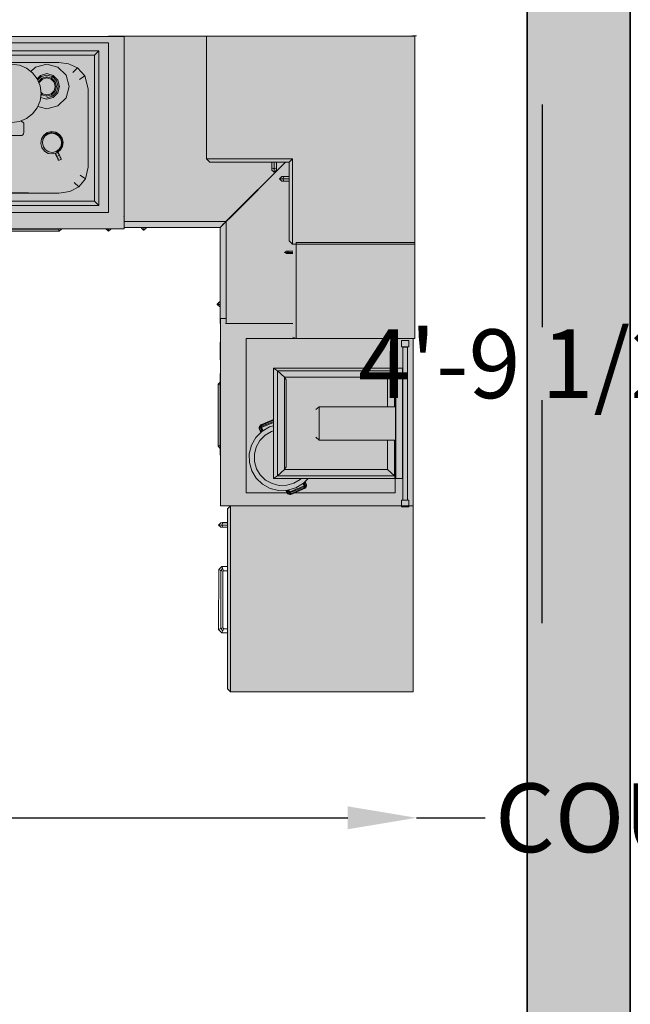
# Model space of a CAD drawing. Units: inches. Extents: x 2178 to 3409, y 1711 to 2279.
# Tile 6 of 8: x 2423 to 2476, y 2140 to 2226. Entities that reach past the tile are written whole.
import ezdxf

# ---------------------------------------------------------------- set-up
doc = ezdxf.new("R2010")
doc.units = ezdxf.units.IN
for name, color, linetype, lineweight in [('A-ANNO-DIMS', 2, 'Continuous', 18), ('A-FLOR-FIXT', 8, 'Continuous', 18), ('A-WALL', 7, 'Continuous', 35), ('A-WALL-PATT', 252, 'Continuous', 13)]:
    doc.layers.add(name, color=color, linetype=linetype, lineweight=lineweight)
doc.layers.add('hatch', color=254, linetype='Continuous')
doc.styles.get("Standard").update_dxf_attribs({"font": 'arial.ttf'})
doc.dimstyles.get("Standard").update_dxf_attribs({"dimtxt": 6, "dimasz": 6, "dimexe": 0.18, "dimexo": 0.0625, "dimgap": 0.09, "dimtad": 0, "dimtih": 1, "dimtoh": 1, "dimdec": 4, "dimzin": 0, "dimdsep": 46, "dimlunit": 4, "dimtxsty": 'Standard', "dimcen": 0.09, "dimse1": 1, "dimse2": 1, "dimadec": 0, "dimazin": 0, "dimtfac": 1, "dimtdec": 4, "dimtofl": 0, "dimtmove": 0, "dimatfit": 3, "dimfxl": 1, "dimtolj": 1, "dimtzin": 0, "dimarcsym": 0})

# ---------------------------------------------------------------- blocks, each defined once
blk = doc.blocks.new('kithen1')
at = {"layer": 'hatch'}
blk.add_hatch(color=256, dxfattribs=at).paths.add_polyline_path([(-2799.7, -8.3), (-2273.3, -8.3), (-2273.3, -1.7), (-2257.5, -1.7), (-2257.5, -1.1), (-1023.7, -1.1), (-1023.7, 0), (0, 0), (0, -0.3), (0.3, -0.3), (0.3, -1009.9), (-6.1, -1009.9), (-6.1, -2189.3), (-615.8, -2189.3), (-626.5, -2178.9), (-626.5, -1578.2), (-615.8, -1567.8), (-649.5, -1567.8), (-649.5, -1399.1), (-650.3, -1399.1), (-650.3, -1376.8), (-657.9, -1368.5), (-657.8, -1162.4), (-650.3, -1155.1), (-650.3, -1126.4), (-649.5, -1126.4), (-649.5, -1081.1), (-650.3, -1081.1), (-650.3, -1021.1), (-649.5, -1021.1), (-649.5, -959.1), (-651, -959.1), (-650.7, -903), (-653.5, -903), (-660.6, -895.5), (-660.5, -894.6), (-653.5, -887.1), (-651, -887.1), (-651, -638.7), (-651.2, -638.5), (-898.3, -638.5), (-898.3, -640.4), (-905.9, -647.4), (-906.8, -647.4), (-914.3, -640.4), (-914.3, -638.5), (-971.4, -638.5), (-971.4, -642.6), (-1016.2, -642.6), (-1016.2, -643.9), (-1023.8, -650.9), (-1024.7, -650.9), (-1032.2, -643.9), (-1032.2, -642.6), (-1179.7, -642.6), (-1188.8, -650.9), (-1395.6, -650.9), (-1403.7, -642.6), (-1813.5, -642.6), (-1822.6, -650.9), (-2029.4, -650.9), (-2037.5, -642.6), (-2257.5, -642.6), (-2257.5, -618.1), (-2261.3, -618.1), (-2271.7, -628.7), (-2458, -628.7), (-2727.7, -628.7), (-2727.7, -651.1), (-2735, -658.1), (-2735.9, -658), (-2743.2, -651.1), (-2743.2, -628.7), (-2789.4, -628.7), (-2799.7, -618.1)])
at = {"color": 0}
for p, q in [((0, 0), (-1023.7, 0)), ((-696.5, 0), (-696.5, -409.2)), ((-8.6, 1.9), (-10.5, 0)), ((-10.1, 0), (-8.2, 1.9)), ((-8.2, 1.9), (-8.3, 1.8)), ((-8.3, 1.9), (-8.3, 0)), ((5.4, 1.8), (-8.3, 1.8)), ((0, 0), (0, -694.7)), ((0, -0.3), (0, 0)), ((-2261.3, -8.3), (-2799.7, -8.3)), ((-2799.7, -8.3), (-2799.7, -618.1)), ((-2273.3, -1.9), (-2273.9, -1.9)), ((-2273.9, -1.9), (-2273.9, -8.3)), ((-2261.3, -1.7), (-2273.3, -1.7)), ((-2273.3, -1.7), (-2273.3, -8.3)), ((-2261.3, -601.6), (-2261.3, -1.7)), ((-2261.3, -618.1), (-2261.3, -8.3)), ((-2261, -8.5), (-2261.3, -8.5)), ((-971.4, -1.1), (-2257.5, -1.1)), ((-2257.5, -1.1), (-2257.5, -642.6)), ((-1023.7, -22.5), (-2210.1, -22.5)), ((-2210.1, -22.5), (-2210.1, -589.1)), ((-1023.7, -589.1), (-1023.7, -22.5)), ((-971.4, -1.1), (-971.4, -600.9)), ((0.3, -0.3), (0, -0.3)), ((0.3, -671.1), (0.3, -0.3)), ((-2257.5, -51.5), (-2261.3, -51.5)), ((-2261.3, -51.5), (-2261.3, -536.3)), ((-2183.7, -48.8), (-1056.9, -48.9)), ((-2169.4, -62.7), (-2183.7, -48.8)), ((-2183.7, -48.8), (-2183.7, -565)), ((-2169.7, -550.2), (-2169.4, -62.7)), ((-1071, -63.6), (-2169.4, -62.7)), ((-1056.9, -48.9), (-1071, -63.6)), ((-1071, -550.2), (-1071, -63.6)), ((-1056.9, -48.9), (-1056.9, -565)), ((-2136.6, -97.6), (-2156.1, -126.2)), ((-2103.6, -76.6), (-2136.6, -97.6)), ((-2135.1, -98.9), (-2102.3, -78.1)), ((-2100.1, -80.6), (-2132.5, -101.2)), ((-2093.2, -88.3), (-2124.5, -108.2)), ((-2057.7, -68.5), (-2103.6, -76.6)), ((-2102.3, -78.1), (-2056.8, -70)), ((-2100.1, -80.6), (-2102.3, -78.1)), ((-2055, -72.6), (-2100.1, -80.6)), ((-2093.2, -88.3), (-2100.1, -80.6)), ((-2049.7, -80.6), (-2093.2, -88.3)), ((-1740.9, -68.5), (-2057.7, -68.5)), ((-2056.8, -70), (-1741.9, -70)), ((-1743.7, -72.6), (-2055, -72.6)), ((-1749, -80.6), (-2049.7, -80.6)), ((-1716.2, -84.8), (-1749, -80.6)), ((-1709.7, -76.9), (-1743.7, -72.6)), ((-1741.9, -70), (-1707.6, -74.4)), ((-1706.4, -72.9), (-1740.9, -68.5)), ((-1685.6, -98.8), (-1716.2, -84.8)), ((-1678, -91.5), (-1709.7, -76.9)), ((-1707.6, -74.4), (-1675.5, -89.1)), ((-1674.1, -87.7), (-1706.4, -72.9)), ((-1678, -91.5), (-1685.6, -98.8)), ((-1651.9, -119.5), (-1678, -91.5)), ((-1675.5, -89.1), (-1649.1, -117.4)), ((-1647.6, -116.2), (-1674.1, -87.7)), ((-1523.7, -95.6), (-1554, -114.9)), ((-1481.5, -88.1), (-1523.7, -95.6)), ((-1523.7, -95.6), (-1509.8, -111.1)), ((-1189.8, -88.1), (-1481.5, -88.1)), ((-1396, -106.6), (-1372.5, -96.9)), ((-1372.5, -96.9), (-1347.3, -93.6)), ((-1347.3, -93.6), (-1322, -96.9)), ((-1322, -96.9), (-1298.5, -106.6)), ((-1268.1, -102.9), (-1230.5, -92.9)), ((-1230.5, -92.9), (-1193, -102.9)), ((-1157.9, -92.2), (-1189.8, -88.1)), ((-1128.2, -105.8), (-1157.9, -92.2)), ((-2156.1, -126.2), (-2163.3, -163.2)), ((-2161.7, -164.1), (-2154.5, -127.3)), ((-2151.7, -129.3), (-2158.8, -165.7)), ((-2154.5, -127.3), (-2135.1, -98.9)), ((-2151.7, -129.3), (-2154.5, -127.3)), ((-2132.5, -101.2), (-2151.7, -129.3)), ((-2143, -135.3), (-2151.7, -129.3)), ((-2124.5, -108.2), (-2143, -135.3)), ((-2132.5, -101.2), (-2135.1, -98.9)), ((-2124.5, -108.2), (-2132.5, -101.2)), ((-1685.6, -98.8), (-1660.4, -125.8)), ((-1660.4, -125.8), (-1651.9, -119.5)), ((-1648.8, -170.4), (-1660.4, -125.8)), ((-1649.1, -117.4), (-1651.9, -119.5)), ((-1651.9, -119.5), (-1639.9, -165.7)), ((-1649.1, -117.4), (-1637, -164.1)), ((-1635.3, -163.2), (-1647.6, -116.2)), ((-1554, -114.9), (-1572, -141.2)), ((-1431.7, -142.2), (-1416.2, -122.1)), ((-1416.2, -122.1), (-1396, -106.6)), ((-1298.5, -106.6), (-1278.3, -122.1)), ((-1283.4, -118.2), (-1268.1, -102.9)), ((-1278.3, -122.1), (-1262.8, -142.2)), ((-1252, -130.7), (-1263.1, -141.8)), ((-1252, -130.7), (-1230.5, -124.9)), ((-1249.5, -134.9), (-1230.5, -129.8)), ((-1230.5, -124.9), (-1209.1, -130.7)), ((-1230.5, -129.8), (-1211.6, -134.9)), ((-1209.1, -130.7), (-1193.4, -146.3)), ((-1193, -102.9), (-1165.5, -130.3)), ((-1165.5, -130.3), (-1155.5, -167.7)), ((-1143.5, -120.5), (-1128.2, -105.8)), ((-1128.2, -105.8), (-1103.8, -132)), ((-2163.3, -163.2), (-2163.3, -447.5)), ((-2161.7, -446.6), (-2161.7, -164.1)), ((-2149.9, -170.5), (-2143, -135.3)), ((-1637, -164.1), (-1637, -446.6)), ((-1635.3, -447.4), (-1635.3, -163.2)), ((-1572, -141.2), (-1578.6, -175.3)), ((-1572, -141.2), (-1554.6, -153.3)), ((-1441.5, -165.7), (-1431.7, -142.2)), ((-1262.8, -142.2), (-1253, -165.7)), ((-1249.5, -134.9), (-1261, -146.4)), ((-1258.4, -151.7), (-1258.6, -152.3)), ((-1246.6, -139.9), (-1258.4, -151.7)), ((-1255.2, -153.5), (-1258.4, -151.7)), ((-1255.2, -153.5), (-1256.4, -157.6)), ((-1244.8, -143), (-1255.2, -153.5)), ((-1230.5, -135.6), (-1246.6, -139.9)), ((-1246.6, -139.9), (-1244.8, -143)), ((-1244.8, -143), (-1230.5, -139.2)), ((-1214.5, -139.9), (-1230.5, -135.6)), ((-1230.5, -135.6), (-1230.5, -139.2)), ((-1230.5, -139.2), (-1216.3, -143)), ((-1216.3, -143), (-1214.5, -139.9)), ((-1205.8, -153.5), (-1216.3, -143)), ((-1211.6, -134.9), (-1214.5, -139.9)), ((-1214.5, -139.9), (-1202.7, -151.7)), ((-1211.6, -134.9), (-1197.7, -148.8)), ((-1202.7, -151.7), (-1205.8, -153.5)), ((-1205.8, -153.5), (-1202, -167.7)), ((-1198.4, -167.7), (-1202.7, -151.7)), ((-1197.7, -148.8), (-1192.6, -167.7)), ((-1193.4, -146.3), (-1187.6, -167.7)), ((-1103.8, -132), (-1120.8, -144.8)), ((-1103.8, -132), (-1092.5, -175.3)), ((-2158.8, -165.7), (-2158.8, -445)), ((-2149.9, -440.2), (-2149.9, -170.5)), ((-1648.8, -440.2), (-1648.8, -170.4)), ((-1639.9, -165.7), (-1639.9, -445)), ((-1578.6, -175.3), (-1578.6, -437)), ((-1444.8, -190.8), (-1441.5, -165.7)), ((-1441.5, -216), (-1444.8, -190.8)), ((-1253, -165.7), (-1249.7, -190.8)), ((-1249.7, -190.8), (-1253, -216)), ((-1250.2, -186.9), (-1244.8, -192.3)), ((-1246.6, -195.5), (-1249.9, -192.2)), ((-1244.8, -192.3), (-1246.6, -195.5)), ((-1230.5, -199.7), (-1246.6, -195.5)), ((-1230.5, -196.1), (-1244.8, -192.3)), ((-1216.3, -192.3), (-1230.5, -196.1)), ((-1214.5, -195.5), (-1230.5, -199.7)), ((-1230.5, -196.1), (-1230.5, -199.7)), ((-1205.8, -181.9), (-1216.3, -192.3)), ((-1216.3, -192.3), (-1214.5, -195.5)), ((-1214.5, -195.5), (-1202.7, -183.7)), ((-1211.6, -200.5), (-1214.5, -195.5)), ((-1197.7, -186.6), (-1211.6, -200.5)), ((-1193.4, -189.1), (-1209.1, -204.7)), ((-1202, -167.7), (-1205.8, -181.9)), ((-1205.8, -181.9), (-1202.7, -183.7)), ((-1202.7, -183.7), (-1198.4, -167.7)), ((-1202, -167.7), (-1198.4, -167.7)), ((-1192.6, -167.7), (-1197.7, -186.6)), ((-1187.6, -167.7), (-1193.4, -189.1)), ((-1155.5, -167.7), (-1165.5, -205.1)), ((-1092.5, -175.3), (-1092.5, -437)), ((-1442, -212), (-1442.1, -213.6)), ((-1442.1, -213.6), (-1441.9, -216.3)), ((-1441.9, -216.3), (-1441.5, -218.2)), ((-1431.7, -239.4), (-1441.5, -216)), ((-1441.5, -218.2), (-1440.8, -218.9)), ((-1440.8, -218.9), (-1440.3, -218.9)), ((-1253, -216), (-1262.8, -239.4)), ((-1230.5, -210.4), (-1251.6, -204.8)), ((-1250.8, -199.1), (-1249.5, -200.5)), ((-1211.6, -200.5), (-1230.5, -205.5)), ((-1209.1, -204.7), (-1230.5, -210.4)), ((-1165.5, -205.1), (-1193, -232.5)), ((-1416.2, -259.6), (-1431.7, -239.4)), ((-1396, -275), (-1416.2, -259.6)), ((-1278.3, -259.6), (-1298.5, -275)), ((-1262.8, -239.4), (-1278.3, -259.6)), ((-1230.5, -242.5), (-1260.7, -234.4)), ((-1193, -232.5), (-1230.5, -242.5)), ((-1914.6, -272.1), (-1926.9, -292)), ((-1926.9, -292), (-1921.4, -314.8)), ((-1891.8, -266.6), (-1914.6, -272.1)), ((-1871.8, -278.8), (-1891.8, -266.6)), ((-1866.3, -301.6), (-1871.8, -278.8)), ((-1493.1, -302.1), (-1453.2, -294.2)), ((-1453.2, -294.3), (-1493.1, -302.2)), ((-1453.2, -294.2), (-1413.4, -302.1)), ((-1413.4, -302.2), (-1453.2, -294.3)), ((-1453.2, -294.3), (-1453.2, -296.5)), ((-1372.5, -284.8), (-1396, -275)), ((-1347.3, -288.1), (-1372.5, -284.8)), ((-1364, -321.4), (-1354.5, -287.1)), ((-1322, -284.8), (-1347.3, -288.1)), ((-1298.5, -275), (-1322, -284.8)), ((-1316.5, -282.5), (-1307.2, -290.8)), ((-1307.2, -290.8), (-1307.2, -321.4)), ((-1921.4, -314.8), (-1901.4, -327)), ((-1901.4, -327), (-1878.5, -321.5)), ((-1878.5, -321.5), (-1866.3, -301.6)), ((-1526.8, -324.6), (-1549.4, -358.3)), ((-1549.4, -358.3), (-1526.8, -324.6)), ((-1525.2, -326.2), (-1547.3, -359.2)), ((-1526.8, -324.6), (-1493.1, -302.1)), ((-1493.1, -302.2), (-1526.8, -324.6)), ((-1492.2, -304.2), (-1525.2, -326.2)), ((-1486.4, -318.2), (-1514.5, -337)), ((-1453.2, -296.5), (-1492.2, -304.2)), ((-1453.2, -311.7), (-1486.4, -318.2)), ((-1453.2, -296.5), (-1414.2, -304.2)), ((-1453.2, -311.7), (-1420.1, -318.2)), ((-1453.2, -338.2), (-1453.2, -311.7)), ((-1420.1, -318.2), (-1392, -337)), ((-1413.4, -302.1), (-1379.6, -324.6)), ((-1379.6, -324.6), (-1413.4, -302.2)), ((-1379.6, -324.6), (-1357, -358.3)), ((-1357, -358.3), (-1379.6, -324.6)), ((-1363.6, -324.3), (-1364, -321.4)), ((-1361.6, -328), (-1363.6, -324.3)), ((-1357.9, -330.6), (-1361.6, -328)), ((-1308.2, -326), (-1310.7, -329.1)), ((-1307.2, -321.4), (-1308.2, -326)), ((-1240.7, -330.6), (-1228.9, -321.9)), ((-1227.6, -324.8), (-1238.3, -332.8)), ((-1236.8, -334.2), (-1226.7, -326.8)), ((-1228.9, -321.9), (-1214.7, -318.4)), ((-1227.6, -324.8), (-1228.3, -323.3)), ((-1214.6, -321.6), (-1227.6, -324.8)), ((-1226.7, -326.8), (-1214.5, -323.7)), ((-1214.7, -318.4), (-1200.3, -320.6)), ((-1214.7, -319.9), (-1214.6, -321.6)), ((-1214.6, -321.6), (-1201.4, -323.6)), ((-1214.5, -323.7), (-1202.1, -325.6)), ((-1202.1, -325.6), (-1191.3, -332)), ((-1201.4, -323.6), (-1200.8, -322)), ((-1201.4, -323.6), (-1189.9, -330.5)), ((-1200.3, -320.6), (-1187.7, -328.1)), ((-1187.7, -328.1), (-1179, -339.8)), ((-1549.4, -358.3), (-1557.3, -398)), ((-1557.3, -398), (-1549.4, -358.3)), ((-1547.3, -359.2), (-1555.1, -398)), ((-1514.5, -337), (-1533.3, -365)), ((-1508.7, -375.1), (-1495.7, -355.7)), ((-1495.7, -355.7), (-1476.2, -342.8)), ((-1476.2, -342.8), (-1453.2, -338.2)), ((-1430.3, -342.8), (-1453.2, -338.2)), ((-1410.8, -355.7), (-1430.3, -342.8)), ((-1397.8, -375.1), (-1410.8, -355.7)), ((-1392, -337), (-1373.2, -365)), ((-1352.7, -331.6), (-1357.9, -330.6)), ((-1357, -358.3), (-1349.1, -398)), ((-1349.1, -398), (-1357, -358.3)), ((-1318.5, -331.6), (-1352.7, -331.6)), ((-1314.3, -331), (-1318.5, -331.6)), ((-1310.7, -329.1), (-1314.3, -331)), ((-1250.4, -357.6), (-1248.3, -343.1)), ((-1246.9, -371.7), (-1250.4, -357.6)), ((-1248.3, -343.1), (-1240.7, -330.6)), ((-1245.1, -357.3), (-1243.2, -344.9)), ((-1242, -369.4), (-1245.1, -357.3)), ((-1243.2, -344.9), (-1236.8, -334.2)), ((-1191.3, -332), (-1183.9, -342.1)), ((-1189.9, -330.5), (-1188.7, -329.2)), ((-1189.9, -330.5), (-1181.9, -341.2)), ((-1183.9, -342.1), (-1180.8, -354.2)), ((-1180.8, -354.2), (-1182.7, -366.6)), ((-1181.9, -341.2), (-1180.4, -340.5)), ((-1181.9, -341.2), (-1178.7, -354.1)), ((-1178.7, -354.1), (-1180.7, -367.3)), ((-1179, -339.8), (-1175.5, -354)), ((-1178.7, -354.1), (-1177, -354.1)), ((-1175.5, -354), (-1177.6, -368.4)), ((-1533.3, -365), (-1539.9, -398)), ((-1513.2, -398), (-1508.7, -375.1)), ((-1393.2, -398), (-1397.8, -375.1)), ((-1373.2, -365), (-1366.6, -398)), ((-1238.2, -383.5), (-1246.9, -371.7)), ((-1234.6, -379.5), (-1242, -369.4)), ((-1225.6, -391), (-1238.2, -383.5)), ((-1223.8, -385.9), (-1234.6, -379.5)), ((-1211.2, -393.1), (-1225.6, -391)), ((-1211.4, -387.8), (-1223.8, -385.9)), ((-1199.2, -384.8), (-1211.4, -387.8)), ((-1197, -389.6), (-1211.2, -393.1)), ((-1202.1, -390.9), (-1202.4, -391)), ((-1202.4, -391), (-1202, -390.9)), ((-1202.4, -391), (-1202.4, -391)), ((-1202.4, -391), (-1202.3, -391.3)), ((-1202.3, -391.3), (-1200.2, -395.7)), ((-1202, -390.9), (-1202.1, -390.9)), ((-1201.7, -390.8), (-1199.7, -395.1)), ((-1199.7, -395.1), (-1198, -394.1)), ((-1189.2, -377.3), (-1199.2, -384.8)), ((-1187.6, -378.8), (-1198.3, -386.7)), ((-1185.2, -380.9), (-1197, -389.6)), ((-1193.3, -386.9), (-1194.2, -387.6)), ((-1193.1, -386.7), (-1193.3, -386.9)), ((-1193.3, -386.9), (-1191.3, -391.2)), ((-1191.3, -391.2), (-1193.2, -391.8)), ((-1192.7, -386.5), (-1192.9, -386.6)), ((-1192.6, -386.8), (-1192.7, -386.5)), ((-1190.5, -391.2), (-1192.6, -386.8)), ((-1191.3, -391.2), (-1190.5, -391.2)), ((-1188.3, -397.5), (-1191.3, -391.2)), ((-1190.5, -391.2), (-1187.6, -397.2)), ((-1182.7, -366.6), (-1189.2, -377.3)), ((-1180.7, -367.3), (-1187.6, -378.8)), ((-1187.6, -378.8), (-1186.3, -379.9)), ((-1177.6, -368.4), (-1185.2, -380.9)), ((-1180.7, -367.3), (-1179.1, -367.9)), ((-1557.3, -398), (-1549.4, -437.8)), ((-1549.4, -437.8), (-1557.3, -398)), ((-1555.1, -398), (-1547.3, -436.9)), ((-1539.9, -398), (-1533.3, -431.1)), ((-1508.7, -420.9), (-1513.2, -398)), ((-1495.7, -440.4), (-1508.7, -420.9)), ((-1410.8, -440.4), (-1397.8, -420.9)), ((-1397.8, -420.9), (-1393.2, -398)), ((-1366.6, -398), (-1373.2, -431.1)), ((-1349.1, -398), (-1357, -437.8)), ((-1357, -437.8), (-1349.1, -398)), ((-1200.2, -395.7), (-1199.7, -395.1)), ((-1200.2, -395.7), (-1197.3, -401.8)), ((-1199.7, -395.1), (-1196.7, -401.5)), ((-1197.3, -401.8), (-1196.7, -401.5)), ((-1197.3, -401.8), (-1194.5, -407.8)), ((-1196.7, -401.5), (-1190.1, -398.4)), ((-1196.7, -401.5), (-1193.7, -407.8)), ((-1194.5, -407.8), (-1193.7, -407.8)), ((-1192.4, -412.2), (-1194.5, -407.8)), ((-1193.7, -407.8), (-1191.8, -407.2)), ((-1193.7, -407.8), (-1191.5, -412.5)), ((-1191.6, -413.9), (-1192.4, -412.2)), ((-1190.7, -414.2), (-1191.6, -413.9)), ((-1188.7, -413.8), (-1190.7, -414.2)), ((-1190.1, -398.4), (-1188.3, -397.5)), ((-1186.2, -412.8), (-1188.7, -413.8)), ((-1187.6, -397.2), (-1188.3, -397.5)), ((-1188.3, -397.5), (-1185.3, -403.9)), ((-1184.8, -403.3), (-1187.6, -397.2)), ((-1185.3, -403.9), (-1186.9, -404.9)), ((-1183.8, -411.5), (-1186.2, -412.8)), ((-1185.3, -403.9), (-1184.8, -403.3)), ((-1183.1, -408.5), (-1185.3, -403.9)), ((-1184.8, -403.3), (-1182.7, -407.7)), ((-1182.3, -410.2), (-1183.8, -411.5)), ((-1182.7, -407.7), (-1181.9, -409.3)), ((-1181.9, -409.3), (-1182.3, -410.2)), ((-696.5, -409.2), (-408.8, -409.2)), ((-685.5, -420.3), (-696.5, -409.2)), ((-419.9, -420.3), (-685.5, -420.3)), ((-432.1, -420.3), (-630.9, -618.1)), ((-630.6, -618.4), (-431.9, -420.3)), ((-614.8, -602.2), (-432.2, -420.3)), ((-431.9, -420.3), (-614.5, -602.5)), ((-432, -420.3), (-607.9, -595.8)), ((-432.1, -420.3), (-607.9, -595.4)), ((-478.5, -420.3), (-478.5, -439.9)), ((-470.7, -443), (-470.7, -420.3)), ((-462.9, -420.3), (-462.9, -439.9)), ((-408.8, -409.2), (-419.9, -420.3)), ((-419.9, -683.7), (-419.9, -420.3)), ((-408.8, -409.2), (-408.8, -694.7)), ((-2163.3, -447.5), (-2159.9, -473.6)), ((-2158.2, -472.6), (-2161.7, -446.6)), ((-2158.8, -445), (-2155.4, -470.7)), ((-2146.6, -465), (-2149.9, -440.2)), ((-1658, -480.4), (-1648.8, -440.2)), ((-1639.9, -445), (-1649.4, -486.6)), ((-1637, -446.6), (-1646.6, -488.6)), ((-1645, -489.8), (-1635.3, -447.4)), ((-1578.6, -437), (-1575.5, -461.1)), ((-1575.5, -461.1), (-1557.8, -449.7)), ((-1549.4, -437.8), (-1526.8, -471.4)), ((-1526.8, -471.4), (-1549.4, -437.8)), ((-1547.3, -436.9), (-1525.2, -469.8)), ((-1533.3, -431.1), (-1514.5, -459.1)), ((-1514.5, -459.1), (-1486.4, -477.9)), ((-1476.2, -453.3), (-1495.7, -440.4)), ((-1453.2, -457.9), (-1476.2, -453.3)), ((-1453.2, -457.9), (-1430.3, -453.3)), ((-1453.2, -484.4), (-1453.2, -457.9)), ((-1430.3, -453.3), (-1410.8, -440.4)), ((-1392, -459.1), (-1420.1, -477.9)), ((-1373.2, -431.1), (-1392, -459.1)), ((-1357, -437.8), (-1379.6, -471.4)), ((-1379.6, -471.4), (-1357, -437.8)), ((-1092.5, -437), (-1101.4, -476)), ((-478.5, -439.9), (-470.7, -443)), ((-478.5, -439.9), (-478.5, -446.8)), ((-478.5, -446.8), (-470.7, -454.1)), ((-462.9, -439.9), (-470.7, -443)), ((-470.7, -443), (-470.7, -454.1)), ((-470.7, -454.1), (-462.9, -446.8)), ((-462.9, -446.8), (-462.9, -439.9)), ((-2159.9, -473.6), (-2141.1, -508.3)), ((-2139.6, -507.1), (-2158.2, -472.6)), ((-2155.4, -470.7), (-2146.6, -465)), ((-2137, -504.8), (-2155.4, -470.7)), ((-2146.6, -465), (-2128.8, -498)), ((-2085.5, -509.3), (-2116.3, -487.4)), ((-2060.9, -482.3), (-2085.5, -509.3)), ((-1680.2, -507.9), (-1658, -480.4)), ((-1649.4, -486.6), (-1672.5, -515.1)), ((-1646.6, -488.6), (-1669.9, -517.4)), ((-1668.5, -518.8), (-1645, -489.8)), ((-1649.4, -486.6), (-1658, -480.4)), ((-1646.6, -488.6), (-1649.4, -486.6)), ((-1575.5, -461.1), (-1558.2, -493)), ((-1558.2, -493), (-1526.7, -515.5)), ((-1493.1, -493.9), (-1526.8, -471.4)), ((-1526.8, -471.4), (-1493.1, -493.9)), ((-1525.2, -469.8), (-1492.2, -491.9)), ((-1492.2, -491.9), (-1453.2, -499.6)), ((-1486.4, -477.9), (-1453.2, -484.4)), ((-1420.1, -477.9), (-1453.2, -484.4)), ((-1453.2, -499.6), (-1414.2, -491.9)), ((-1379.6, -471.4), (-1413.4, -493.9)), ((-1413.4, -493.9), (-1379.6, -471.4)), ((-1123, -502.7), (-1138.7, -488.2)), ((-1101.4, -476), (-1123, -502.7)), ((-1101.4, -476), (-1118.7, -463.5)), ((-444.9, -468.4), (-452.2, -476.2)), ((-452.2, -476.2), (-441.1, -476.2)), ((-452.2, -476.2), (-444.9, -484)), ((-419.9, -468.4), (-444.9, -468.4)), ((-444.9, -484), (-438, -484)), ((-441.1, -476.2), (-438, -468.4)), ((-419.9, -476.2), (-441.1, -476.2)), ((-441.1, -476.2), (-438, -484)), ((-438, -484), (-419.9, -484)), ((-2141.1, -508.3), (-2106.9, -532.7)), ((-2137, -504.8), (-2139.6, -507.1)), ((-2105.6, -531.3), (-2139.6, -507.1)), ((-2128.8, -498), (-2137, -504.8)), ((-2103.3, -528.8), (-2137, -504.8)), ((-2128.8, -498), (-2096.3, -521.1)), ((-2096.3, -521.1), (-2103.3, -528.8)), ((-2096.3, -521.1), (-2085.5, -509.3)), ((-2049.7, -530.1), (-2096.3, -521.1)), ((-2085.5, -509.3), (-2041.5, -517.8)), ((-1711.5, -524.5), (-1749, -530.1)), ((-1680.2, -507.9), (-1711.5, -524.5)), ((-1672.5, -515.1), (-1704.9, -532.3)), ((-1702.7, -534.9), (-1669.9, -517.4)), ((-1668.5, -518.8), (-1701.5, -536.3)), ((-1672.5, -515.1), (-1680.2, -507.9)), ((-1669.9, -517.4), (-1672.5, -515.1)), ((-1189.8, -524.2), (-1668.5, -518.8)), ((-1481.5, -524.2), (-1668.5, -518.8)), ((-1526.7, -515.5), (-1512.6, -500.1)), ((-1526.7, -515.5), (-1481.5, -524.2)), ((-1453.2, -501.8), (-1493.1, -493.9)), ((-1493.1, -493.9), (-1453.2, -501.8)), ((-1189.8, -524.2), (-1481.5, -524.2)), ((-1413.4, -493.9), (-1453.2, -501.8)), ((-1453.2, -501.8), (-1413.4, -493.9)), ((-1453.2, -499.6), (-1453.2, -501.8)), ((-1153.4, -518.8), (-1189.8, -524.2)), ((-1123, -502.7), (-1153.4, -518.8)), ((-2257.5, -535.3), (-2257.9, -535.3)), ((-2183.7, -565), (-2169.7, -550.2)), ((-1793.1, -550.2), (-2169.7, -550.2)), ((-2106.9, -532.7), (-2057.7, -542.2)), ((-2103.3, -528.8), (-2105.6, -531.3)), ((-2056.8, -540.7), (-2105.6, -531.3)), ((-2055, -538.1), (-2103.3, -528.8)), ((-2057.7, -542.2), (-2056.8, -540.7)), ((-1783.5, -542.2), (-2057.7, -542.2)), ((-1781.7, -540.7), (-2056.8, -540.7)), ((-1778.6, -538.1), (-2055, -538.1)), ((-1749, -530.1), (-2049.7, -530.1)), ((-1749, -530.1), (-1797.1, -530.1)), ((-1743.7, -538.1), (-1797.1, -538.1)), ((-1741.9, -540.7), (-1797.1, -540.7)), ((-1740.9, -542.2), (-1797.1, -542.2)), ((-1071, -550.2), (-1797.1, -550.2)), ((-1704.9, -532.3), (-1743.7, -538.1)), ((-1741.9, -540.7), (-1702.7, -534.9)), ((-1740.9, -542.2), (-1741.9, -540.7)), ((-1701.5, -536.3), (-1740.9, -542.2)), ((-1056.9, -565), (-1071, -550.2)), ((-540.1, -527.9), (-540.1, -528.1)), ((-2210.1, -589.1), (-1789.4, -589.1)), ((-1797.1, -565), (-2183.7, -565)), ((-1056.9, -565), (-1797.1, -565)), ((-1797.1, -589.1), (-1023.7, -589.1)), ((-597, -584.5), (-597, -584.9)), ((-2799.7, -618.1), (-2261.3, -618.1)), ((-2789.4, -628.7), (-2799.7, -618.1)), ((-2261.3, -618.1), (-2271.7, -628.7)), ((-2261, -596.4), (-2261.3, -596.4)), ((-2261.3, -626.3), (-2261.3, -601.6)), ((-972.7, -601.6), (-972.7, -603)), ((-971.4, -600.6), (-971.4, -601.6)), ((-971.4, -603), (-971.4, -642.6)), ((-630.9, -618.1), (-971.4, -618.1)), ((-611.6, -599.1), (-651.2, -638.5)), ((-611.6, -599.4), (-651, -638.7)), ((-642.6, -629.8), (-630.9, -618.1)), ((-630.6, -618.4), (-642.3, -630.1)), ((-630.9, -618.1), (-614.8, -602.2)), ((-614.5, -602.5), (-630.6, -618.4)), ((-630.6, -959.1), (-630.6, -618.4)), ((-620.1, -607.7), (-609.4, -597.1)), ((-619.9, -607.6), (-620.1, -607.6)), ((-620.1, -607.9), (-620.1, -607.7)), ((-609, -596.9), (-609.4, -596.9)), ((-609.4, -597.1), (-609.4, -597.2)), ((-607.9, -595.4), (-607.9, -595.8)), ((-2271.7, -628.7), (-2789.4, -628.7)), ((-2743.2, -628.7), (-2743.2, -644.8)), ((-2743.2, -644.8), (-2742.3, -644.5)), ((-2743.2, -651.1), (-2743.2, -644.8)), ((-2742.3, -650.3), (-2743.2, -651.1)), ((-2742.3, -651.1), (-2743.2, -651.1)), ((-2743.2, -651.1), (-2735.9, -658)), ((-2742.3, -628.7), (-2742.3, -644.4)), ((-2742.3, -644.4), (-2734.9, -647.4)), ((-2742.3, -644.4), (-2742.3, -651.1)), ((-2735, -658.1), (-2742.3, -651.1)), ((-2734.9, -647.4), (-2735, -658.1)), ((-2735, -658.1), (-2727.7, -651.1)), ((-2734.9, -647.4), (-2734.9, -628.7)), ((-2727.7, -644.4), (-2734.9, -647.4)), ((-2727.7, -628.7), (-2727.7, -644.4)), ((-2727.7, -651.1), (-2727.7, -644.4)), ((-2679.7, -628.7), (-2679.4, -647.7)), ((-2679.4, -647.7), (-2665.9, -642)), ((-2669.5, -658), (-2679.4, -647.7)), ((-2666.7, -651.1), (-2672.6, -644.8)), ((-2666.7, -651.1), (-2669.5, -658)), ((-2663.9, -644.2), (-2666.7, -651.1)), ((-2472.3, -651.1), (-2666.7, -651.1)), ((-2665.6, -628.7), (-2665.9, -642)), ((-2665.9, -642), (-2663.9, -644.2)), ((-2663.9, -644.2), (-2474.9, -644.1)), ((-2474.9, -644.1), (-2471.7, -641.3)), ((-2474.9, -644.1), (-2472.3, -651.1)), ((-2472.3, -651.1), (-2465, -644.4)), ((-2469.7, -658.1), (-2472.3, -651.1)), ((-2471.7, -641.3), (-2472, -628.7)), ((-2458.4, -647.4), (-2471.7, -641.3)), ((-2458.4, -647.4), (-2469.7, -658.1)), ((-2458, -628.7), (-2458.4, -647.4)), ((-2261.3, -643.6), (-2261.3, -626.3)), ((-2257.5, -642.6), (-1797.1, -642.6)), ((-2037.5, -642.6), (-2029.4, -650.9)), ((-2029.4, -650.9), (-2026.5, -643.9)), ((-2029.4, -650.9), (-1828.9, -650.9)), ((-2026.5, -643.9), (-2027.8, -642.6)), ((-2025.9, -642.6), (-2026.5, -643.9)), ((-2026.5, -643.9), (-1828.9, -643.9)), ((-1825.3, -643.9), (-1828.9, -643.9)), ((-1822.6, -650.9), (-1828.9, -650.9)), ((-1825.8, -642.6), (-1825.3, -643.9)), ((-1825.3, -643.9), (-1823.8, -642.6)), ((-1822.6, -650.9), (-1825.3, -643.9)), ((-1813.5, -642.6), (-1822.6, -650.9)), ((-971.4, -642.6), (-1797.1, -642.6)), ((-1395.6, -650.9), (-1403.7, -642.6)), ((-1392.7, -643.9), (-1395.6, -650.9)), ((-1395.6, -650.9), (-1188.8, -650.9)), ((-1394, -642.6), (-1392.7, -643.9)), ((-1392.7, -643.9), (-1392.1, -642.6)), ((-1191.5, -643.9), (-1392.7, -643.9)), ((-1192, -642.6), (-1191.5, -643.9)), ((-1191.5, -643.9), (-1190, -642.6)), ((-1188.8, -650.9), (-1191.5, -643.9)), ((-1179.7, -642.6), (-1188.8, -650.9)), ((-1032.2, -643.9), (-1032.2, -642.6)), ((-1031.4, -643.1), (-1032.2, -643.9)), ((-1031.4, -643.9), (-1032.2, -643.9)), ((-1032.2, -643.9), (-1024.7, -650.9)), ((-1031.4, -642.6), (-1031.4, -643.9)), ((-1023.8, -650.9), (-1031.4, -643.9)), ((-1024.7, -650.9), (-1023.8, -650.9)), ((-1023.8, -650.9), (-1023.8, -642.6)), ((-1016.2, -643.9), (-1023.8, -650.9)), ((-1016.2, -642.6), (-1016.2, -643.9)), ((-971.4, -635.7), (-971.4, -641.8)), ((-971.4, -641.8), (-971.4, -638.3)), ((-651.2, -638.5), (-971.4, -638.5)), ((-914.3, -640.4), (-914.4, -638.5)), ((-913.5, -639.6), (-914.3, -640.4)), ((-913.5, -640.4), (-914.3, -640.4)), ((-914.3, -640.4), (-906.8, -647.3)), ((-913.5, -638.5), (-913.5, -640.4)), ((-905.9, -647.4), (-913.5, -640.4)), ((-906.8, -647.3), (-905.9, -647.4)), ((-905.9, -647.4), (-905.9, -638.5)), ((-898.3, -640.4), (-905.9, -647.4)), ((-898.3, -638.5), (-898.3, -640.4)), ((-651, -638.7), (-651, -959.1)), ((-2735.9, -658), (-2735, -658.1)), ((-2669.5, -658), (-2469.7, -658.1)), ((-408.8, -694.7), (-419.9, -683.7)), ((-0.1, -689.2), (-397.2, -689.2)), ((-397.2, -689.2), (-397.2, -1009.9)), ((-0.1, -1009.9), (-0.1, -689.2)), ((0, -694.7), (0, -671.1)), ((0, -671.1), (0.3, -671.1)), ((-429, -718.2), (-436, -721.9)), ((-436, -721.9), (-425.3, -721.9)), ((-436, -721.9), (-429, -725.7)), ((-407.9, -718.2), (-429, -718.2)), ((-425.3, -721.9), (-422.2, -718.2)), ((-407.9, -721.9), (-425.3, -721.9)), ((-425.3, -721.9), (-422.2, -725.7)), ((0, -694.7), (-408.8, -694.7)), ((-0.1, -699.8), (-0.1, -998.7)), ((0.3, -700.4), (-0.1, -700.4)), ((0.3, -998.7), (0.3, -700.4)), ((-429, -725.7), (-422.2, -725.7)), ((-422.2, -725.7), (-407.9, -725.7)), ((-660.5, -894.6), (-653.5, -887.1)), ((-651, -887), (-653.5, -887.1)), ((-653.5, -887.1), (-652.7, -887.9)), ((-653.5, -887.1), (-653.5, -887.9)), ((-653.5, -887.9), (-660.6, -895.5)), ((-660.6, -895.5), (-660.5, -894.6)), ((-660.6, -895.5), (-651, -895.5)), ((-653.5, -903), (-660.6, -895.5)), ((-653.5, -887.9), (-651, -887.9)), ((-651, -903), (-653.5, -903)), ((-633.4, -942.7), (-649.5, -942.7)), ((-649.5, -942.7), (-649.5, -1567.8)), ((-651, -959.1), (-649.5, -959.1)), ((-630.6, -959.1), (-633.4, -959.1)), ((-407.9, -959.1), (-630.6, -959.1)), ((-398.5, -1009.2), (-564.1, -1009.2)), ((-564.1, -1009.2), (-564.1, -1525)), ((-397.2, -1009.9), (-407.9, -1004.5)), ((-397.2, -1009.9), (-0.1, -1009.9)), ((-65.6, -1009.9), (-65.6, -1108.4)), ((-20.3, -1015.5), (-44.8, -1015.5)), ((-44.8, -1015.5), (-44.8, -1037.5)), ((-20.3, -1037.5), (-20.3, -1015.5)), ((-6.1, -1009.9), (-6.1, -1567.8)), ((-0.1, -998.7), (0.3, -998.7)), ((-649.5, -1021.1), (-650.3, -1021.1)), ((-650.3, -1021.1), (-650.3, -1081.1)), ((-44.8, -1037.5), (-20.3, -1037.5)), ((-24.8, -1038), (-40.6, -1038)), ((-40.6, -1038), (-40.6, -1549.4)), ((-24.8, -1549.4), (-24.8, -1038)), ((-650.3, -1081.1), (-649.5, -1081.1)), ((-62.5, -1108.4), (-473.1, -1108.4)), ((-473.1, -1108.4), (-459.2, -1117.2)), ((-473.1, -1108.4), (-473.1, -1476.7)), ((-459.2, -1117.2), (-68.2, -1117.2)), ((-459.2, -1467.9), (-459.2, -1117.2)), ((-459.2, -1117.2), (-435.9, -1138.2)), ((-91.6, -1138.2), (-68.2, -1117.2)), ((-68.2, -1117.2), (-67.2, -1115.5)), ((-68.2, -1117.2), (-68.2, -1237.1)), ((-64.1, -1108.4), (-67.2, -1111.2)), ((-67.2, -1111.2), (-67.2, -1237.1)), ((-40.9, -1108.4), (-64.1, -1108.4)), ((-64.1, -1108.4), (-64.1, -1476.7)), ((-40.9, -1476.7), (-40.9, -1108.4)), ((-649.5, -1126.4), (-650.3, -1126.4)), ((-650.3, -1126.4), (-650.3, -1186.4)), ((-435.9, -1138.2), (-91.6, -1138.2)), ((-435.9, -1138.2), (-430.1, -1147)), ((-435.9, -1447), (-435.9, -1138.2)), ((-430.1, -1147), (-430.1, -1438.2)), ((-91.6, -1138.2), (-91.6, -1237.1)), ((-657.8, -1162.4), (-657.9, -1368.5)), ((-650.3, -1155.1), (-657.8, -1162.4)), ((-657.8, -1162.4), (-650.8, -1165.4)), ((-650.8, -1165.4), (-650.3, -1164.8)), ((-650.8, -1365.8), (-650.8, -1165.4)), ((-650.8, -1165.4), (-650.3, -1165.6)), ((-650.3, -1186.4), (-649.5, -1186.4)), ((-649.5, -1231.7), (-650.3, -1231.7)), ((-650.3, -1231.7), (-650.3, -1291.7)), ((-320.2, -1237.1), (-330.5, -1246.3)), ((-64.3, -1237.1), (-320.2, -1237.1)), ((-320.2, -1237.1), (-320.2, -1348.4)), ((-64.3, -1348.4), (-64.3, -1237.1)), ((-473.1, -1280.2), (-515, -1298.2)), ((-473.1, -1282.1), (-514, -1299.7)), ((-650.3, -1291.7), (-649.5, -1291.7)), ((-519.1, -1303.5), (-520.1, -1306.8)), ((-520.1, -1306.8), (-520.1, -1310.2)), ((-520.1, -1310.2), (-514.9, -1323)), ((-517.4, -1300.6), (-519.1, -1303.5)), ((-517.7, -1304.5), (-518.6, -1307.4)), ((-518.6, -1307.4), (-518.6, -1310.5)), ((-518.6, -1310.5), (-513.9, -1322)), ((-516.2, -1301.9), (-517.7, -1304.5)), ((-515.4, -1308), (-517.7, -1304.5)), ((-515, -1298.2), (-517.4, -1300.6)), ((-514, -1299.7), (-516.2, -1301.9)), ((-515.4, -1308), (-516.2, -1301.9)), ((-514, -1299.7), (-515.4, -1308)), ((-512, -1302.3), (-515.4, -1308)), ((-515.4, -1308), (-512.4, -1308.2)), ((-511.2, -1319.3), (-515.4, -1308)), ((-512, -1302.3), (-514, -1299.7)), ((-511.2, -1305.5), (-512.4, -1308.2)), ((-512.4, -1308.2), (-511.3, -1307.8)), ((-512.4, -1308.2), (-508, -1317.5)), ((-512.4, -1308.2), (-508.5, -1317.7)), ((-508.7, -1317.8), (-512.4, -1308.2)), ((-473.1, -1286.3), (-512, -1302.3)), ((-511.2, -1305.5), (-512, -1302.3)), ((-486.2, -1304.5), (-511.4, -1319.5)), ((-511.3, -1307.8), (-510.4, -1305.8)), ((-511.3, -1307.8), (-507.6, -1317.2)), ((-473.1, -1289.8), (-511.2, -1305.5)), ((-510.4, -1305.8), (-511.2, -1305.5)), ((-473.1, -1290.3), (-510.4, -1305.8)), ((-473.1, -1300.7), (-486.2, -1304.5)), ((-649.5, -1339.1), (-650.3, -1339.1)), ((-650.3, -1339.1), (-650.3, -1399.1)), ((-531.9, -1340.4), (-546.3, -1365.8)), ((-511.4, -1319.5), (-531.9, -1340.4)), ((-500.9, -1332.7), (-518.2, -1350.4)), ((-479.5, -1319.9), (-500.9, -1332.7)), ((-473.1, -1318.1), (-479.5, -1319.9)), ((-320.2, -1348.4), (-330.5, -1339.2)), ((-657.9, -1368.5), (-650.8, -1365.8)), ((-657.9, -1368.5), (-650.3, -1376.8)), ((-650.3, -1365.6), (-650.8, -1365.8)), ((-650.8, -1365.8), (-650.3, -1366.5)), ((-546.3, -1365.8), (-553.5, -1394)), ((-530.4, -1372), (-536.6, -1395.8)), ((-518.2, -1350.4), (-530.4, -1372)), ((-320.2, -1348.4), (-64.3, -1348.4)), ((-91.6, -1447), (-91.6, -1348.4)), ((-68.2, -1348.4), (-68.2, -1467.9)), ((-67.2, -1474), (-67.2, -1348.4)), ((-650.3, -1399.1), (-649.5, -1399.1)), ((-553.5, -1394), (-553.2, -1423)), ((-536.6, -1395.8), (-536.3, -1420.4)), ((-553.2, -1423), (-545.3, -1450.9)), ((-536.3, -1420.4), (-529.6, -1444.1)), ((-529.6, -1444.1), (-516.9, -1465.1)), ((-430.1, -1438.2), (-435.9, -1447)), ((-545.3, -1450.9), (-530.3, -1475.7)), ((-530.3, -1475.7), (-509.3, -1495.8)), ((-516.9, -1465.1), (-499.1, -1482.2)), ((-473.1, -1476.7), (-459.2, -1467.9)), ((-162.2, -1476.7), (-473.1, -1476.7)), ((-473.1, -1476.7), (-64.1, -1476.7)), ((-435.9, -1447), (-459.2, -1467.9)), ((-459.2, -1467.9), (-68.2, -1467.9)), ((-91.6, -1447), (-435.9, -1447)), ((-383.1, -1479.8), (-380.1, -1476.7)), ((-372.5, -1493), (-356.6, -1476.7)), ((-68.2, -1467.9), (-91.6, -1447)), ((-68.2, -1467.9), (-67.2, -1469.6)), ((-64.1, -1476.7), (-67.2, -1474)), ((-65.6, -1476.7), (-65.6, -1525)), ((-64.1, -1476.7), (-40.9, -1476.7)), ((-509.3, -1495.8), (-483.7, -1509.8)), ((-499.1, -1482.2), (-477.4, -1494)), ((-483.7, -1509.8), (-455.3, -1516.7)), ((-477.4, -1494), (-453.3, -1499.9)), ((-453.3, -1499.9), (-428.4, -1499.4)), ((-428.4, -1499.4), (-404.5, -1492.5)), ((-426, -1516.1), (-397.7, -1508)), ((-371, -1502.5), (-418.6, -1522)), ((-371.9, -1502.2), (-417.9, -1521.4)), ((-417.7, -1525.2), (-370.2, -1505.7)), ((-368.3, -1508.3), (-414.8, -1528.3)), ((-367.2, -1509.7), (-414.4, -1530.1)), ((-404.5, -1492.5), (-383.1, -1479.8)), ((-397.7, -1508), (-372.5, -1493)), ((-371, -1500.1), (-373.6, -1493.6)), ((-373, -1493.3), (-369.9, -1499.8)), ((-369.9, -1499.8), (-372.7, -1493.1)), ((-372.5, -1493), (-369.9, -1499.8)), ((-371, -1500.1), (-371.9, -1502.2)), ((-371.9, -1502.2), (-371, -1502.5)), ((-371, -1502.5), (-369.9, -1499.8)), ((-369.9, -1499.8), (-371, -1500.1)), ((-370.2, -1505.7), (-371, -1502.5)), ((-366.9, -1500), (-370.3, -1490.7)), ((-366.9, -1500), (-370.2, -1505.7)), ((-370.2, -1505.7), (-368.3, -1508.3)), ((-369.9, -1499.8), (-366.9, -1500)), ((-368.3, -1508.3), (-366.9, -1500)), ((-366.1, -1506.1), (-368.3, -1508.3)), ((-367.6, -1488), (-363.7, -1497.5)), ((-364.8, -1507.3), (-367.2, -1509.7)), ((-364.5, -1503.5), (-366.9, -1500)), ((-366.9, -1500), (-366.1, -1506.1)), ((-366.6, -1486.9), (-362.2, -1497.8)), ((-366.1, -1506.1), (-364.5, -1503.5)), ((-363.1, -1504.4), (-364.8, -1507.3)), ((-363.7, -1500.6), (-364.5, -1503.5)), ((-363.7, -1497.5), (-363.7, -1500.6)), ((-362.2, -1501.2), (-363.1, -1504.4)), ((-362.2, -1497.8), (-362.2, -1501.2)), ((-564.1, -1525), (-426.8, -1525)), ((-455.3, -1516.7), (-426, -1516.1)), ((-426.6, -1525.5), (-430.8, -1516.2)), ((-429.6, -1516.2), (-425.8, -1524.2)), ((-424.2, -1527.8), (-426.6, -1525.5)), ((-423.4, -1522.1), (-426.1, -1516.1)), ((-425.8, -1524.2), (-423.6, -1526.3)), ((-421.2, -1529.4), (-424.2, -1527.8)), ((-423.6, -1526.3), (-423.4, -1522.1)), ((-420.9, -1527.8), (-423.6, -1526.3)), ((-420.8, -1520.4), (-423.4, -1522.1)), ((-423.4, -1522.1), (-417.7, -1525.2)), ((-420.8, -1520.4), (-423.3, -1515.3)), ((-422.4, -1515.1), (-419.6, -1520.1)), ((-419.6, -1520.1), (-421.9, -1514.9)), ((-417.9, -1530.2), (-421.2, -1529.4)), ((-417.7, -1525.2), (-420.9, -1527.8)), ((-420.9, -1527.8), (-418, -1528.4)), ((-419.6, -1520.1), (-420.8, -1520.4)), ((-418.6, -1522), (-420.8, -1520.4)), ((-417.9, -1521.4), (-419.6, -1520.1)), ((-418.6, -1522), (-417.9, -1521.4)), ((-417.7, -1525.2), (-418.6, -1522)), ((-418, -1528.4), (-414.8, -1528.3)), ((-414.4, -1530.1), (-417.9, -1530.2)), ((-414.8, -1528.3), (-417.7, -1525.2)), ((-65.6, -1525), (-402.7, -1525)), ((-44.8, -1567.8), (-649.5, -1567.8)), ((-626.5, -1578.2), (-615.8, -1567.8)), ((-626.5, -2178.9), (-626.5, -1578.2)), ((-6.1, -1567.8), (-615.8, -1567.8)), ((-615.8, -1567.8), (-615.8, -2189.3)), ((-20.3, -1549.4), (-44.8, -1549.4)), ((-44.8, -1549.4), (-44.8, -1571.3)), ((-44.8, -1571.3), (-20.3, -1571.3)), ((-20.3, -1571.3), (-20.3, -1549.4)), ((-6.1, -1567.8), (-20.3, -1567.8)), ((-6.1, -2189.3), (-6.1, -1567.8)), ((-655.9, -1632.5), (-648.9, -1625.2)), ((-655.8, -1631.6), (-655.9, -1632.5)), ((-645.2, -1632.6), (-655.9, -1632.5)), ((-655.9, -1632.5), (-648.9, -1639.8)), ((-648.9, -1624.4), (-655.8, -1631.6)), ((-648.9, -1624.4), (-642.6, -1624.3)), ((-648.9, -1625.2), (-648.9, -1624.4)), ((-648.1, -1625.2), (-648.9, -1624.4)), ((-642.1, -1625.2), (-648.9, -1625.2)), ((-648.9, -1639.8), (-642.1, -1639.8)), ((-642.1, -1625.2), (-645.2, -1632.6)), ((-642.1, -1639.8), (-645.2, -1632.6)), ((-645.2, -1632.6), (-626.5, -1632.6)), ((-626.5, -1624.3), (-642.6, -1624.3)), ((-642.6, -1624.3), (-642.3, -1625.2)), ((-626.5, -1625.2), (-642.1, -1625.2)), ((-626.5, -1639.8), (-642.1, -1639.8)), ((-655.8, -1781), (-645.4, -1771.2)), ((-626.5, -1770.8), (-645.4, -1771.2)), ((-645.4, -1771.2), (-639.8, -1784.7)), ((-655.8, -1781), (-655.9, -1980.9)), ((-648.9, -1783.9), (-655.8, -1781)), ((-648.9, -1783.9), (-642.6, -1777.9)), ((-641.9, -1786.7), (-648.9, -1783.9)), ((-648.9, -1978.3), (-648.9, -1783.9)), ((-639.8, -1784.7), (-641.9, -1786.7)), ((-641.9, -1786.7), (-641.8, -1975.6)), ((-626.5, -1785), (-639.8, -1784.7)), ((-655.9, -1980.9), (-648.9, -1978.3)), ((-645.2, -1992.2), (-655.9, -1980.9)), ((-641.8, -1975.6), (-648.9, -1978.3)), ((-648.9, -1978.3), (-642.1, -1985.5)), ((-645.2, -1992.2), (-639.1, -1978.9)), ((-626.5, -1992.6), (-645.2, -1992.2)), ((-641.8, -1975.6), (-639.1, -1978.9)), ((-639.1, -1978.9), (-626.5, -1978.6)), ((-626.5, -2178.9), (-615.8, -2189.3)), ((-615.8, -2189.3), (-6.1, -2189.3))]:
    blk.add_line(p, q, dxfattribs=at)
blk.add_lwpolyline([(-2799.7, -8.3), (-2273.3, -8.3), (-2273.3, -1.7), (-2257.5, -1.7), (-2257.5, -1.1), (-1023.7, -1.1), (-1023.7, 0), (0, 0), (0, -0.3), (0.3, -0.3), (0.3, -1009.9), (-6.1, -1009.9), (-6.1, -2189.3), (-615.8, -2189.3), (-626.5, -2178.9), (-626.5, -1578.2), (-615.8, -1567.8), (-649.5, -1567.8), (-649.5, -1399.1), (-650.3, -1399.1), (-650.3, -1376.8), (-657.9, -1368.5), (-657.8, -1162.4), (-650.3, -1155.1), (-650.3, -1126.4), (-649.5, -1126.4), (-649.5, -1081.1), (-650.3, -1081.1), (-650.3, -1021.1), (-649.5, -1021.1), (-649.5, -959.1), (-651, -959.1), (-650.7, -903), (-653.5, -903), (-660.6, -895.5), (-660.5, -894.6), (-653.5, -887.1), (-651, -887.1), (-651, -638.7), (-651.2, -638.5), (-898.3, -638.5), (-898.3, -640.4), (-905.9, -647.4), (-906.8, -647.4), (-914.3, -640.4), (-914.3, -638.5), (-971.4, -638.5), (-971.4, -642.6), (-1016.2, -642.6), (-1016.2, -643.9), (-1023.8, -650.9), (-1024.7, -650.9), (-1032.2, -643.9), (-1032.2, -642.6), (-1179.7, -642.6), (-1188.8, -650.9), (-1395.6, -650.9), (-1403.7, -642.6), (-1813.5, -642.6), (-1822.6, -650.9), (-2029.4, -650.9), (-2037.5, -642.6), (-2257.5, -642.6), (-2257.5, -618.1), (-2261.3, -618.1), (-2271.7, -628.7), (-2458, -628.7), (-2727.7, -628.7), (-2727.7, -651.1), (-2735, -658.1), (-2735.9, -658), (-2743.2, -651.1), (-2743.2, -628.7), (-2789.4, -628.7), (-2799.7, -618.1), (-2799.7, -8.3)])
blk = doc.blocks.new('*D21')
at = {"layer": 'A-ANNO-DIMS', "color": 0, "lineweight": -2, "transparency": 16777216}
for p, q in [((2502.613, 2232.043), (2502.613, 2175.145)), ((2502.613, 2112.043), (2502.613, 2168.94))]:
    blk.add_line(p, q, dxfattribs=at)
at = {"layer": 'A-ANNO-DIMS', "color": 0, "transparency": 16777216}
for points in [[(2501.613, 2232.043), (2503.613, 2232.043), (2502.613, 2238.043)], [(2501.613, 2112.043), (2503.613, 2112.043), (2502.613, 2106.043)]]:
    blk.add_solid(points, dxfattribs=at)
at = {"layer": 'Defpoints', "color": 0, "transparency": 16777216}
for p in [(2467.065, 2238.043), (2467.065, 2106.043), (2502.613, 2106.043)]:
    blk.add_point(p, dxfattribs=at)
at = {"layer": 'A-ANNO-DIMS', "color": 0, "transparency": 16777216, "insert": (2502.613, 2172.043), "char_height": 6, "attachment_point": 5}
blk.add_mtext("\\A1;11'", dxfattribs=at)
blk = doc.blocks.new('*D57')
at = {"layer": 'A-ANNO-DIMS', "color": 0, "lineweight": -2, "transparency": 16777216}
for p, q in [((2390.072, 2155.967), (2451.379, 2155.967)), ((2457.379, 2155.967), (2463.379, 2155.967))]:
    blk.add_line(p, q, dxfattribs=at)
at = {"layer": 'A-ANNO-DIMS', "color": 0, "transparency": 16777216}
for points in [[(2390.072, 2156.967), (2390.072, 2154.967), (2384.072, 2155.967)], [(2451.379, 2156.967), (2451.379, 2154.967), (2457.379, 2155.967)]]:
    blk.add_solid(points, dxfattribs=at)
at = {"layer": 'Defpoints', "color": 0, "transparency": 16777216}
for p in [(2384.072, 2166.963), (2457.379, 2166.963), (2457.379, 2155.967)]:
    blk.add_point(p, dxfattribs=at)
at = {"layer": 'A-ANNO-DIMS', "color": 0, "transparency": 16777216, "insert": (2500.286, 2155.967), "char_height": 6, "attachment_point": 5}
blk.add_mtext('\\A1;COUNTER 6\'-1 1/2"', dxfattribs=at)
blk = doc.blocks.new('*D58')
at = {"layer": 'A-ANNO-DIMS', "color": 0, "lineweight": -2, "transparency": 16777216}
for p, q in [((2468.375, 2218.227), (2468.375, 2198.787)), ((2468.375, 2172.963), (2468.375, 2192.403))]:
    blk.add_line(p, q, dxfattribs=at)
at = {"layer": 'A-ANNO-DIMS', "color": 0, "transparency": 16777216}
for points in [[(2467.375, 2218.227), (2469.375, 2218.227), (2468.375, 2224.227)], [(2467.375, 2172.963), (2469.375, 2172.963), (2468.375, 2166.963)]]:
    blk.add_solid(points, dxfattribs=at)
at = {"layer": 'Defpoints', "color": 0, "transparency": 16777216}
for p in [(2457.379, 2224.227), (2468.375, 2224.227), (2457.379, 2166.963)]:
    blk.add_point(p, dxfattribs=at)
at = {"layer": 'A-ANNO-DIMS', "color": 0, "transparency": 16777216, "insert": (2468.375, 2195.595), "char_height": 6, "attachment_point": 5}
blk.add_mtext('\\A1;4\'-9 1/2"', dxfattribs=at)

msp = doc.modelspace()

# ---------------------------------------------------------------- hatches: boundary and pattern name
at = {"layer": 'A-WALL-PATT'}
h = msp.add_hatch(color=256, dxfattribs=at)
h.dxf.hatch_style = 1
h.paths.add_polyline_path([(2233.06485, 1992.04256), (2317.06485, 1992.04256), (2317.06485, 1998.04256), (2317.06485, 2006.75072), (2311.06485, 2006.75072), (2311.06485, 1998.04256), (2233.06485, 1998.04256), (2233.06485, 2009.64251), (2224.06485, 2009.64251), (2224.06485, 1863.04256), (2233.06485, 1863.04256), (2278.65041, 1863.04256), (2278.65041, 1872.04256), (2233.06485, 1872.04256)])
h.paths.add_polyline_path([(2359.06485, 1992.04256), (2359.06485, 1998.04256), (2353.06485, 1998.04256), (2353.06485, 1962.04256), (2353.06485, 1872.04256), (2314.65041, 1872.04256), (2314.65041, 1863.04256), (2359.06485, 1863.04256), (2359.06485, 1872.04256)])
h.paths.add_polyline_path([(2401.06485, 1890.04256), (2371.06485, 1890.04256), (2359.06485, 1890.04256), (2359.06485, 1884.04256), (2371.06485, 1884.04256), (2377.06485, 1884.04256), (2401.06485, 1884.04256)])
h.paths.add_polyline_path([(2353.06485, 1802.77269), (2359.06485, 1802.77269), (2359.06485, 1808.77269), (2356.83755, 1808.77269), (2353.06485, 1808.77269), (2347.91295, 1808.77269), (2347.91295, 1802.77269), (2347.91295, 1749.04256), (2342.02347, 1749.04256), (2342.02347, 1743.04256), (2353.06485, 1743.04256)])
h.paths.add_polyline_path([(2476.06485, 2247.04256), (2442.91353, 2247.04256), (2442.91353, 2238.04256), (2467.06485, 2238.04256), (2467.06485, 2041.93675), (2476.06485, 2041.93675)])
h.paths.add_polyline_path([(2467.06485, 2106.04256), (2406.56133, 2106.04256, -0.04188649), (2407.06485, 2100.04256), (2467.06485, 2100.04256)])
h.paths.add_polyline_path([(2406.91353, 2247.04256), (2321.22384, 2247.04256), (2321.22384, 2238.04256), (2365.06485, 2238.04256), (2365.06485, 2106.04256), (2365.06485, 2100.04256), (2371.06485, 2100.04256), (2371.06485, 2136.04256), (2371.06485, 2238.04256), (2406.91353, 2238.04256)])
h.paths.add_polyline_path([(2285.22384, 2247.04256), (2224.06485, 2247.04256), (2224.06485, 2087.1459), (2233.06485, 2087.1459), (2233.06485, 2100.04256), (2329.06485, 2100.04256, -0.04188649), (2329.56837, 2106.04256), (2233.06485, 2106.04256), (2233.06485, 2238.04256), (2285.22384, 2238.04256)])
h.paths.add_polyline_path([(2317.06485, 2052.04256), (2317.06485, 2061.5418), (2311.06485, 2061.5418), (2311.06485, 2052.04256), (2233.06485, 2052.04256), (2233.06485, 2063.1459), (2224.06485, 2063.1459), (2224.06485, 2033.64251), (2233.06485, 2033.64251), (2233.06485, 2046.04256), (2311.06485, 2046.04256), (2311.06485, 2036.1446, -0.05038204), (2317.06485, 2036.75072), (2317.06485, 2046.04256)])

# ---------------------------------------------------------------- linework, layer by layer
at = {"layer": 'A-WALL'}
for p, q in [((2476.06485, 2247.04256), (2476.06485, 1803.04256)), ((2467.06485, 2238.04256), (2467.06485, 1812.04256))]:
    msp.add_line(p, q, dxfattribs=at)

# ---------------------------------------------------------------- block references
at = {"layer": 'A-FLOR-FIXT', "xscale": 0.0261336107367163, "yscale": 0.0261336107367163, "zscale": 0.0261336107367163}
msp.add_blockref('kithen1', (2457.23906, 2224.17699), dxfattribs=at)

# ---------------------------------------------------------------- dimensions: what is measured, and where the dimension line sits
at = {"layer": 'A-ANNO-DIMS'}
for base, p1, p2, override, picture, middle in [((2502.61341, 2106.04256), (2467.06485, 2238.04256), (2467.06485, 2106.04256), {"dimclrd": 0, "dimclre": 0, "dimclrt": 0}, '*D21', (2502.61341, 2172.04256)), ((2468.3751, 2224.22693), (2457.37908, 2166.96329), (2457.37908, 2224.22693), {"dimdec": 1, "dimlfac": 1, "dimrnd": 0, "dimzin": 1, "dimdsep": 46, "dimlunit": 4, "dimfrac": 2}, '*D58', (2468.3751, 2195.59511))]:
    dim = msp.add_linear_dim(base=base, p1=p1, p2=p2, angle=90, dimstyle='Standard', override=override, dxfattribs=at)
    dim.commit()
    dim.dimension.update_dxf_attribs({"geometry": picture, "text_midpoint": middle})
dim = msp.add_linear_dim(base=(2457.37908, 2155.96728), p1=(2384.07233, 2166.96329), p2=(2457.37908, 2166.96329), text='COUNTER <>', dimstyle='Standard', override={"dimdec": 1, "dimlfac": 1, "dimrnd": 0, "dimzin": 1, "dimdsep": 46, "dimlunit": 4, "dimfrac": 2}, dxfattribs=at)
dim.commit()
dim.dimension.update_dxf_attribs({"geometry": '*D57', "text_midpoint": (2500.28559, 2155.96728)})

doc.saveas('drawing.dxf')
